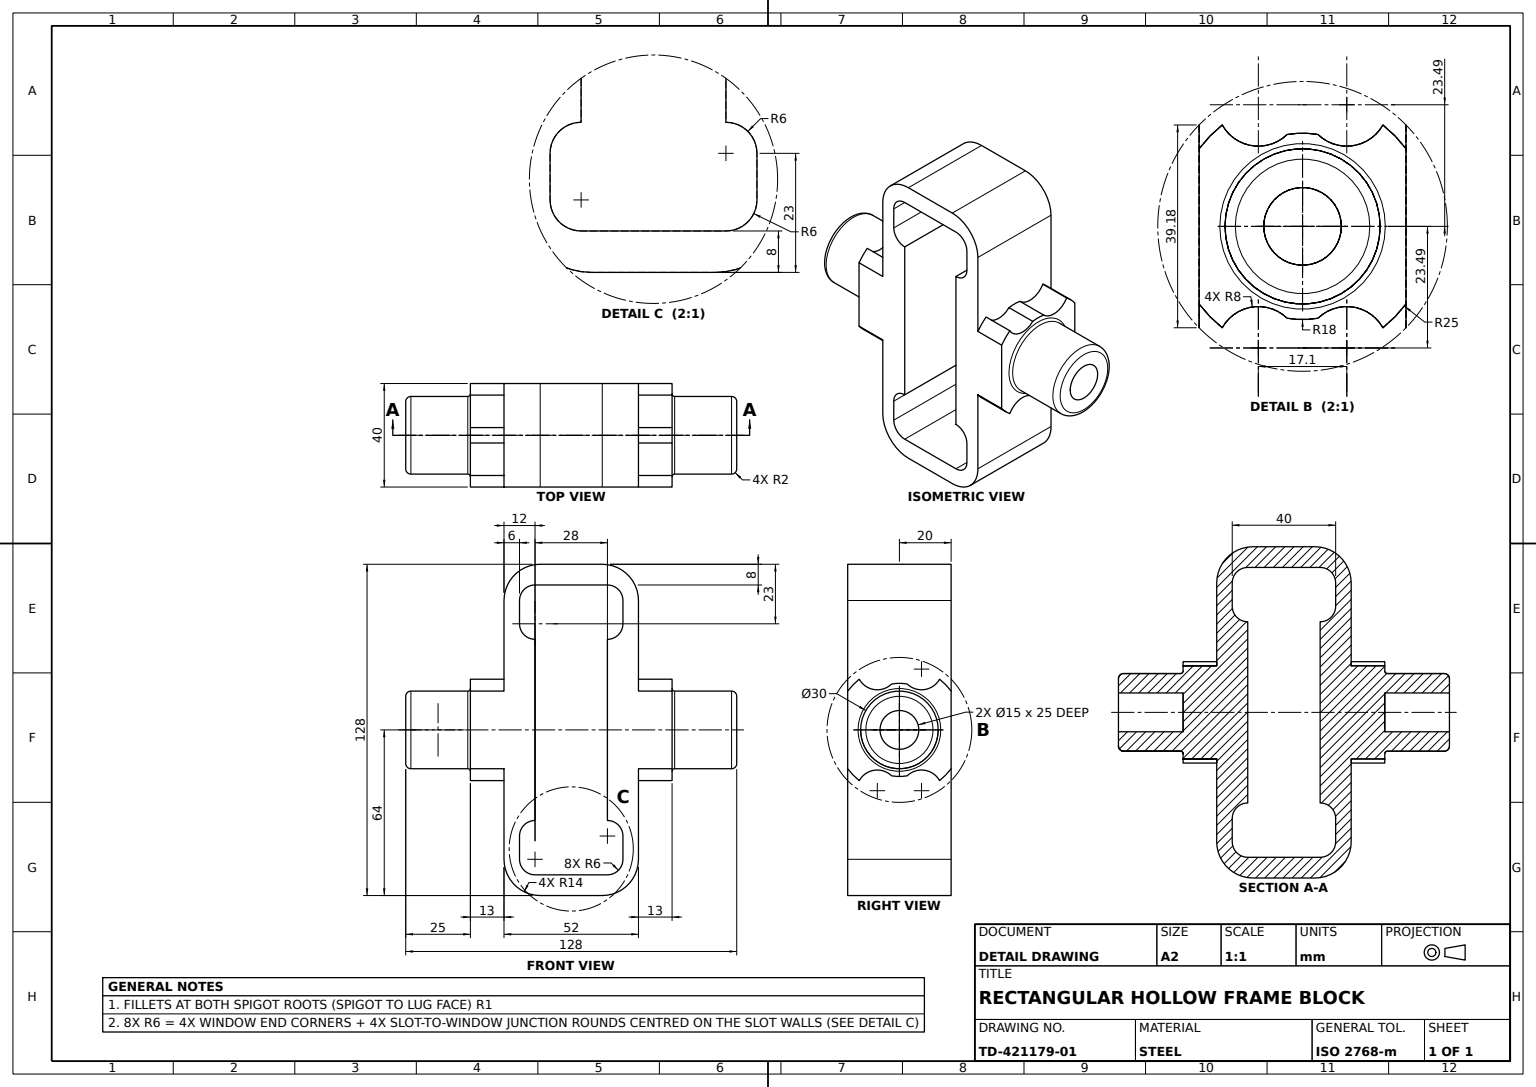
SolidWorks part; units mm, degrees
material "Plain Carbon Steel"
ref_plane "Front Plane" through (0, 0, 0) normal (0, 0, 1) x (1, 0, 0)
ref_plane "Top Plane" through (0, 0, 0) normal (0, 1, 0) x (1, 0, 0)
ref_plane "Right Plane" through (0, 0, 0) normal (1, 0, 0) x (0, 0, -1)
sketch "Frame Profile Sketch" plane through (0, 0, 0) normal (0, 0, 1) x (1, 0, 0)
  line L1 (-12, -64) -> (12, -64)
  line L2 (-26, -50) -> (-26, 50)
  line L3 (-12, 64) -> (12, 64)
  line L4 (26, -50) -> (26, 50)
  line L5 (-26, -64) -> (26, 64) construction
  line L6 (-26, 64) -> (26, -64) construction
  arc A0 (26, -50) -> (12, -64) centre (12, -50) cw
  arc A1 (-12, -64) -> (-26, -50) centre (-12, -50) cw
  arc A2 (12, 64) -> (26, 50) centre (12, 50) cw
  arc A3 (-26, 50) -> (-12, 64) centre (-12, 50) cw
  point P0 (0, 0)
  dimension "D3" = 14
  dimension "D1" = 128
  dimension "D2" = 52
extrude "Frame Body" add sketch "Frame Profile Sketch" along normal blind 40
sketch "Frame Window Sketch" plane through (0, 0, 40) normal (0, 0, 1) x (1, 0, 0)
  line L0 (14, -35) -> (14, 35)
  line L1 (-14, -56) -> (14, -56)
  line L2 (-20, -50) -> (-20, -41)
  line L3 (-14, 56) -> (14, 56)
  line L4 (20, -50) -> (20, -41)
  line L5 (-20, -56) -> (20, 56) construction
  line L6 (-20, 56) -> (20, -56) construction
  line L7 (12, 64) -> (-12, 64) construction
  line L8 (-14, -35) -> (-14, 35)
  line L10 (20, 41) -> (20, 50)
  line L11 (-20, 41) -> (-20, 50)
  arc A0 (-20, 41) -> (-14, 35) centre (-14, 41) ccw
  arc A1 (20, 41) -> (14, 35) centre (14, 41) cw
  arc A2 (14, -35) -> (20, -41) centre (14, -41) cw
  arc A3 (-20, -41) -> (-14, -35) centre (-14, -41) cw
  arc A4 (20, 50) -> (14, 56) centre (14, 50) ccw
  arc A5 (-20, 50) -> (-14, 56) centre (-14, 50) cw
  arc A6 (20, -50) -> (14, -56) centre (14, -50) cw
  arc A7 (-14, -56) -> (-20, -50) centre (-14, -50) cw
  point P0 (0, 0)
  point P5 (0, 0)
  dimension "D11" = 6
  dimension "D12" = 6
  dimension "D13" = 6
  dimension "D14" = 6
  dimension "D15" = 6
  dimension "D1" = 40
  dimension "D2" = 8
  dimension "D3" = 70
  dimension "D6" = 21
  dimension "D4" = 14
  dimension "D5" = 35
  dimension "D7" = 70
  dimension "D8" = 21
  dimension "D9" = 14
  dimension "D10" = 35
extrude "Frame Window Cut" cut sketch "Frame Window Sketch" against normal blind 40
sketch "Side Lug A Sketch" plane through (26, 0, 0) normal (1, 0, 0) x (0, 0, -1)
  line L2 (-40, 15) -> (-40, -15)
  line L4 (0, 15) -> (0, -15)
  line L9 (-40, 50) -> (0, 50) construction
  arc A0 (-17.0215, 17.7519) -> (-22.9785, 17.7519) centre (-20, 0) ccw
  arc A1 (-35.5334, 19.5886) -> (-40, 15) centre (-20, 0) ccw
  arc A2 (-35.5334, 19.5886) -> (-22.9785, 17.7519) centre (-28.5505, 23.4923) ccw
  arc A3 (-17.0215, 17.7519) -> (-4.4666, 19.5886) centre (-11.4495, 23.4923) ccw
  arc A4 (-22.9785, -17.7519) -> (-35.5334, -19.5886) centre (-28.5505, -23.4923) ccw
  arc A5 (-4.4666, -19.5886) -> (-17.0215, -17.7519) centre (-11.4495, -23.4923) ccw
  arc A6 (0, 15) -> (-4.4666, 19.5886) centre (-20, 0) ccw
  arc A7 (-22.9785, -17.7519) -> (-17.0215, -17.7519) centre (-20, 0) ccw
  arc A8 (-40, -15) -> (-35.5334, -19.5886) centre (-20, 0) ccw
  arc A9 (-4.4666, -19.5886) -> (0, -15) centre (-20, 0) ccw
  dimension "D5" = 36
  dimension "D8" = 50
  dimension "D9" = 16
  dimension "D10" = 16
  dimension "D13" = 2
  dimension "D2" = 40
  dimension "D3" = 25
  dimension "D4" = 23.4923
  dimension "D6" = 20
  dimension "D7" = 50
  dimension "D11" = 17.101
  dimension "D12" = 11.4495
  dimension "D14" = 23.4923
  dimension "D15" = 28.5505
  dimension "D16" = 25
  dimension "D17" = 15
extrude "Side Lug A" add sketch "Side Lug A Sketch" along normal blind 13
sketch "Spigot A Sketch" plane through (39, 0, 0) normal (1, 0, 0) x (0, 0, -1)
  circle A0 centre (-20, 0) radius 15
  circle A1 centre (-20, 0) radius 7.5
  dimension "D1" = 30
  dimension "D2" = 15
extrude "Spigot A Ø30" add sketch "Spigot A Sketch" along normal blind 25
sketch "Side Lug B Sketch" plane through (-26, 0, 0) normal (-1, 0, 0) x (0, 0, 1)
  line L0 (0, 50) -> (0, -50) construction
  line L4 (0, 15) -> (0, -15)
  line L5 (40, 15) -> (40, -15)
  arc A0 (4.4666, 19.5886) -> (0, 15) centre (20, 0) ccw
  arc A1 (17.0215, -17.7519) -> (22.9785, -17.7519) centre (20, 0) ccw
  arc A2 (22.9785, 17.7519) -> (35.5334, 19.5886) centre (28.5505, 23.4923) ccw
  arc A3 (4.4666, 19.5886) -> (17.0215, 17.7519) centre (11.4495, 23.4923) ccw
  arc A4 (35.5334, -19.5886) -> (22.9785, -17.7519) centre (28.5505, -23.4923) ccw
  arc A5 (17.0215, -17.7519) -> (4.4666, -19.5886) centre (11.4495, -23.4923) ccw
  arc A6 (0, -15) -> (4.4666, -19.5886) centre (20, 0) ccw
  arc A8 (22.9785, 17.7519) -> (17.0215, 17.7519) centre (20, 0) ccw
  arc A10 (35.5334, -19.5886) -> (40, -15) centre (20, 0) ccw
  arc A11 (40, 15) -> (35.5334, 19.5886) centre (20, 0) ccw
  dimension "D1" = 50
  dimension "D4" = 36
  dimension "D7" = 16
  dimension "D8" = 16
  dimension "D10" = 36.9732
  dimension "D2" = 20
  dimension "D3" = 0
  dimension "D5" = 23.4923
  dimension "D6" = 28.5505
  dimension "D9" = 25
  dimension "D12" = 23.4923
  dimension "D13" = 28.5505
  dimension "D14" = 25
  dimension "D16" = 17.0215
  dimension "D17" = 34.5886
  dimension "D18" = 19.5886
  dimension "D11" = 2
extrude "Side Lug B" add sketch "Side Lug B Sketch" along normal blind 13
sketch "Spigot B Sketch" plane through (-39, 0, 0) normal (-1, 0, 0) x (0, 0, 1)
  circle A0 centre (20, 0) radius 15
  circle A1 centre (20, 0) radius 7.5
  dimension "D1" = 0
  dimension "D2" = 30
  dimension "D4" = 15
  dimension "D3" = 20
extrude "Spigot B Ø30" add sketch "Spigot B Sketch" along normal blind 25
fillet "Spigot Edge Fillets R2" radius 2 2 edges at (-64, 0, 35) (64, 0, 5)
fillet "Lug Blend Fillets R1" radius 1 2 edges at (39, 0, 5) (-39, 0, 35)
